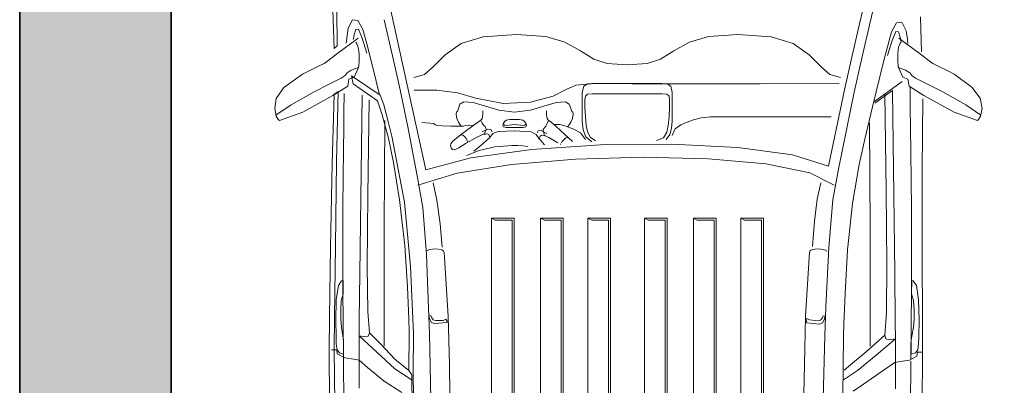
# Model space of a CAD drawing. Units: inches. Extents: x -5 to 482, y -460 to 66.
# Tile 7 of 31: x 33 to 91, y -351 to -329. Entities that reach past the tile are written whole.
import ezdxf

# ---------------------------------------------------------------- set-up
doc = ezdxf.new("R2010")
doc.units = ezdxf.units.IN
doc.header["$MEASUREMENT"] = 0
for name, color, linetype, lineweight in [('A-EQPM-VEHI', 8, 'Continuous', 13), ('A-WALL', 7, 'Continuous', 35), ('A-WALL-PATT', 152, 'Continuous', 13)]:
    doc.layers.add(name, color=color, linetype=linetype, lineweight=lineweight)

msp = doc.modelspace()

# ---------------------------------------------------------------- hatches: boundary and pattern name
at = {"layer": 'A-WALL-PATT'}
h = msp.add_hatch(color=256, dxfattribs=at)
h.dxf.hatch_style = 1
h.paths.add_polyline_path([(149.377, -412.849), (144.377, -412.849), (144.377, -283.849), (144.377, -279.349), (133.877, -279.349), (133.877, -283.849), (139.877, -283.849), (139.877, -412.849), (133.51, -412.849), (133.51, -413.916), (102.652, -413.916), (102.652, -421.02), (133.51, -421.02), (133.51, -421.849), (149.377, -421.849)])
h.paths.add_polyline_path([(226.054, -412.849), (218.877, -412.849), (218.877, -350.849), (262.877, -350.849), (262.877, -386.849), (267.377, -386.849), (267.377, -283.849), (270.377, -283.849), (270.377, -279.349), (244.877, -279.349), (244.877, -283.849), (262.877, -283.849), (262.877, -346.349), (218.877, -346.349), (218.877, -283.849), (220.877, -283.849), (220.877, -279.349), (214.377, -279.349), (214.377, -283.849), (214.377, -412.849), (209.377, -412.849), (209.377, -421.849), (226.054, -421.849)])
h.paths.add_polyline_path([(315.815, -412.849), (250.054, -412.849), (250.054, -421.849), (315.815, -421.849)])
h.paths.add_polyline_path([(430.377, -378.349), (421.377, -378.349), (421.377, -412.849), (375.815, -412.849), (375.815, -421.849), (430.377, -421.849)])
h.paths.add_polyline_path([(78.691, -413.916), (47.68, -413.916), (47.68, -412.849), (41.877, -412.849), (41.877, -283.849), (109.877, -283.849), (109.877, -279.349), (41.877, -279.349), (41.877, -241.849), (32.877, -241.849), (32.877, -421.849), (47.68, -421.849), (47.68, -421.02), (78.691, -421.02)])
h.paths.add_polyline_path([(41.877, -144.349), (154.377, -144.349), (154.377, -137.849), (149.877, -137.849), (149.877, -139.849), (41.877, -139.849), (41.877, -97.849), (32.877, -97.849), (32.877, -181.849), (41.877, -181.849)])
h.paths.add_polyline_path([(430.377, -241.849), (421.377, -241.849), (421.377, -279.349), (309.377, -279.349), (309.377, -170.349), (304.877, -170.349), (304.877, -279.349), (294.377, -279.349), (294.377, -283.849), (421.377, -283.849), (421.377, -318.349), (430.377, -318.349)])
h.paths.add_polyline_path([(430.377, -119.849), (421.377, -119.849), (421.377, -139.849), (419.377, -139.849), (419.377, -144.349), (421.377, -144.349), (421.377, -181.849), (430.377, -181.849)])
h.paths.add_polyline_path([(395.377, -139.849), (377.377, -139.849), (377.377, -75.849), (421.377, -75.849), (421.377, -95.849), (430.377, -95.849), (430.377, -45.599), (421.377, -45.599), (421.377, -71.349), (377.377, -71.349), (377.377, -22.849), (372.877, -22.849), (372.877, -139.849), (242.877, -139.849), (242.877, -137.849), (238.377, -137.849), (238.377, -144.349), (304.877, -144.349), (304.877, -146.349), (309.377, -146.349), (309.377, -144.349), (395.377, -144.349)])
h.paths.add_polyline_path([(65.877, 13.151), (32.877, 13.151), (32.877, -37.849), (41.877, -37.849), (41.877, 4.151), (65.877, 4.151)])
h.paths.add_polyline_path([(166.377, 13.151), (125.877, 13.151), (125.877, 4.151), (149.877, 4.151), (149.877, -113.849), (154.377, -113.849), (154.377, 4.151), (166.377, 4.151)])
h.paths.add_polyline_path([(277.877, 13.151), (226.377, 13.151), (226.377, 4.151), (238.377, 4.151), (238.377, -113.849), (242.877, -113.849), (242.877, 4.151), (277.877, 4.151)])
h.paths.add_polyline_path([(430.377, 13.151), (337.877, 13.151), (337.877, 4.151), (372.877, 4.151), (372.877, 1.151), (377.377, 1.151), (377.377, 4.151), (421.377, 4.151), (421.377, -21.599), (430.377, -21.599)])

# ---------------------------------------------------------------- linework, layer by layer
at = {"layer": 'A-EQPM-VEHI'}
for p, q in [((51.501, -329.276), (51.446, -328.108)), ((54.877, -328.542), (56.991, -338.198)), ((82.759, -329.511), (82.972, -328.603)), ((83.612, -328.412), (83.382, -329.41)), ((51.711, -328.752), (51.727, -330.829)), ((86.365, -329.094), (86.429, -331.173)), ((51.545, -330.986), (51.501, -329.276)), ((52.377, -329.78), (52.336, -330.066)), ((52.377, -329.78), (52.648, -329.267)), ((52.648, -329.267), (52.956, -329.307)), ((52.956, -329.307), (53.25, -329.847)), ((54.521, -329.266), (55.012, -331.413)), ((82.301, -331.49), (82.759, -329.511)), ((83.382, -329.41), (82.89, -331.556)), ((84.946, -329.451), (84.653, -329.99)), ((85.255, -329.411), (84.946, -329.451)), ((85.526, -329.923), (85.255, -329.411)), ((52.969, -330.36), (51.685, -331.319)), ((52.301, -330.358), (52.27, -330.656)), ((52.336, -330.066), (52.301, -330.358)), ((52.744, -330.168), (52.693, -330.377)), ((52.847, -329.847), (52.744, -330.168)), ((53.005, -329.824), (52.847, -329.847)), ((53.215, -330.362), (53.005, -329.824)), ((53.485, -331.257), (53.215, -330.362)), ((53.25, -329.847), (53.492, -330.702)), ((59.102, -330.69), (60.395, -330.28)), ((60.395, -330.28), (62.381, -330.141)), ((62.381, -330.141), (64.123, -330.258)), ((64.123, -330.258), (65.258, -330.594)), ((72.65, -330.594), (73.785, -330.258)), ((73.785, -330.258), (75.527, -330.141)), ((75.527, -330.141), (77.513, -330.28)), ((77.513, -330.28), (78.806, -330.69)), ((84.653, -329.99), (84.177, -331.772)), ((84.688, -330.505), (84.898, -329.968)), ((84.898, -329.968), (85.056, -329.99)), ((85.056, -329.99), (85.159, -330.311)), ((85.089, -330.36), (86.373, -331.319)), ((85.159, -330.311), (85.21, -330.52)), ((85.526, -329.923), (85.562, -330.172)), ((85.562, -330.172), (85.593, -330.425)), ((51.727, -330.829), (51.545, -330.986)), ((52.693, -330.377), (52.679, -330.451)), ((52.835, -330.595), (52.887, -330.666)), ((52.887, -330.666), (52.984, -330.893)), ((52.984, -330.893), (53.036, -331.3)), ((53.492, -330.702), (53.846, -332.115)), ((58.141, -331.359), (59.102, -330.69)), ((65.258, -330.594), (66.182, -331.125)), ((71.727, -331.125), (72.65, -330.594)), ((78.806, -330.69), (79.767, -331.359)), ((84.418, -331.401), (84.688, -330.505)), ((85.075, -330.893), (85.022, -331.3)), ((85.172, -330.666), (85.075, -330.893)), ((85.224, -330.595), (85.172, -330.666)), ((85.21, -330.52), (85.224, -330.595)), ((85.593, -330.425), (85.621, -330.682)), ((51.685, -331.319), (51.096, -331.763)), ((53.036, -331.3), (53.028, -331.733)), ((55.012, -331.413), (55.466, -333.44)), ((57.427, -332.063), (58.141, -331.359)), ((66.182, -331.125), (66.981, -331.617)), ((70.927, -331.617), (71.727, -331.125)), ((79.767, -331.359), (80.481, -332.063)), ((81.864, -333.428), (82.301, -331.49)), ((85.022, -331.3), (85.031, -331.733)), ((86.373, -331.319), (86.963, -331.763)), ((50.669, -332.009), (50.101, -332.288)), ((50.954, -331.871), (50.669, -332.009)), ((51.096, -331.763), (50.954, -331.871)), ((53.003, -332.106), (52.57, -332.273)), ((53.003, -332.106), (52.734, -332.677)), ((53.011, -332.009), (53.003, -332.106)), ((53.028, -331.733), (53.011, -332.009)), ((53.846, -332.115), (54.237, -333.736)), ((56.914, -332.535), (57.427, -332.063)), ((66.981, -331.617), (67.763, -331.878)), ((67.763, -331.878), (68.954, -331.955)), ((68.954, -331.955), (70.145, -331.878)), ((70.145, -331.878), (70.927, -331.617)), ((80.481, -332.063), (80.995, -332.535)), ((82.89, -331.556), (82.436, -333.584)), ((84.177, -331.772), (83.529, -334.456)), ((85.031, -331.733), (85.047, -332.009)), ((85.047, -332.009), (85.056, -332.106)), ((85.056, -332.106), (85.325, -332.677)), ((85.056, -332.106), (85.489, -332.273)), ((86.963, -331.763), (87.104, -331.871)), ((87.104, -331.871), (87.389, -332.008)), ((87.389, -332.008), (87.958, -332.287)), ((49.678, -332.509), (48.571, -333.307)), ((50.101, -332.288), (49.678, -332.509)), ((52.197, -332.576), (51.974, -332.745)), ((52.316, -332.432), (52.197, -332.576)), ((52.57, -332.273), (52.316, -332.432)), ((52.734, -332.677), (52.432, -332.811)), ((52.573, -332.611), (54.277, -333.756)), ((52.69, -333.08), (52.573, -332.611)), ((56.293, -332.697), (56.914, -332.535)), ((80.995, -332.535), (81.616, -332.697)), ((85.325, -332.677), (85.627, -332.811)), ((85.489, -332.273), (85.742, -332.432)), ((85.742, -332.432), (85.862, -332.576)), ((85.862, -332.576), (86.085, -332.745)), ((87.958, -332.287), (88.381, -332.509)), ((88.381, -332.509), (89.411, -333.269)), ((51.223, -333.114), (50.367, -333.56)), ((51.58, -332.944), (51.223, -333.114)), ((51.482, -333.765), (52.365, -333.214)), ((51.974, -332.745), (51.58, -332.944)), ((52.365, -333.214), (52.432, -332.811)), ((54.121, -334.081), (52.69, -333.08)), ((65.908, -333.15), (65.338, -333.419)), ((67.024, -333.06), (65.908, -333.15)), ((66.369, -333.212), (66.285, -333.597)), ((66.587, -333.077), (66.369, -333.212)), ((66.89, -333.061), (66.587, -333.077)), ((71.018, -333.061), (66.89, -333.061)), ((69.258, -333.072), (67.024, -333.06)), ((72.651, -333.079), (69.258, -333.072)), ((71.321, -333.077), (71.018, -333.061)), ((71.539, -333.212), (71.321, -333.077)), ((71.623, -333.597), (71.539, -333.212)), ((76.859, -333.078), (72.651, -333.079)), ((81.536, -333.067), (76.859, -333.078)), ((85.291, -332.946), (83.645, -334.121)), ((85.694, -333.214), (85.627, -332.811)), ((86.577, -333.765), (85.694, -333.214)), ((85.749, -333.232), (85.762, -334.455)), ((86.085, -332.745), (86.479, -332.944)), ((86.479, -332.944), (86.836, -333.114)), ((86.836, -333.114), (87.691, -333.56)), ((89.411, -333.269), (89.915, -333.933)), ((48.571, -333.307), (48.105, -333.952)), ((50.367, -333.56), (48.996, -334.324)), ((49.695, -334.768), (51.482, -333.765)), ((51.438, -337.84), (51.545, -333.691)), ((51.545, -333.691), (51.792, -333.543)), ((51.792, -333.543), (51.695, -337.715)), ((52.141, -333.662), (52.13, -334.738)), ((53.221, -333.746), (53.134, -339.877)), ((54.277, -333.756), (54.505, -334.336)), ((55.466, -333.44), (55.941, -335.733)), ((57.641, -333.457), (56.294, -333.457)), ((58.87, -333.613), (57.641, -333.457)), ((59.974, -333.925), (58.87, -333.613)), ((64.553, -333.821), (63.206, -334.171)), ((65.338, -333.419), (64.553, -333.821)), ((66.285, -333.597), (66.285, -335.29)), ((66.468, -333.818), (66.432, -334.037)), ((66.601, -333.701), (66.468, -333.818)), ((66.873, -333.666), (66.601, -333.701)), ((66.873, -333.666), (71.036, -333.666)), ((71.036, -333.666), (71.307, -333.701)), ((71.307, -333.701), (71.441, -333.818)), ((71.441, -333.818), (71.476, -334.037)), ((71.623, -335.29), (71.623, -333.597)), ((81.522, -335.051), (81.864, -333.428)), ((82.436, -333.584), (81.99, -335.718)), ((83.652, -334.237), (84.705, -333.476)), ((84.25, -333.684), (84.335, -339.434)), ((84.705, -333.476), (84.788, -339.678)), ((88.363, -334.768), (86.577, -333.765)), ((87.691, -333.56), (89.062, -334.324)), ((48.105, -333.952), (48.029, -334.547)), ((48.996, -334.324), (48.096, -334.95)), ((53.638, -334.031), (53.555, -339.704)), ((54.395, -334.921), (54.121, -334.081)), ((54.505, -334.336), (54.786, -335.391)), ((58.935, -334.555), (59.023, -334.293)), ((59.023, -334.293), (59.257, -334.156)), ((59.257, -334.156), (59.799, -334.193)), ((59.799, -334.193), (60.543, -334.402)), ((61.588, -334.25), (59.974, -333.925)), ((60.543, -334.402), (61.335, -334.646)), ((63.206, -334.171), (61.588, -334.25)), ((63.995, -334.402), (63.203, -334.646)), ((64.739, -334.193), (63.995, -334.402)), ((65.282, -334.156), (64.739, -334.193)), ((65.516, -334.293), (65.282, -334.156)), ((65.603, -334.555), (65.516, -334.293)), ((66.432, -334.037), (66.442, -334.464)), ((71.476, -334.037), (71.467, -334.464)), ((83.529, -334.456), (83.074, -336.371)), ((85.762, -334.455), (85.773, -335.747)), ((86.509, -333.977), (86.463, -338.174)), ((89.062, -334.324), (89.963, -334.95)), ((89.915, -333.933), (90.03, -334.547)), ((48.029, -334.547), (48.113, -334.998)), ((48.113, -334.998), (48.235, -335.203)), ((48.297, -335.252), (49.695, -334.768)), ((52.13, -334.738), (52.127, -335.745)), ((54.624, -335.731), (54.395, -334.921)), ((58.789, -334.884), (58.819, -334.749)), ((58.828, -335.143), (58.789, -334.884)), ((58.819, -334.749), (58.87, -334.719)), ((58.87, -334.719), (58.935, -334.555)), ((60.377, -334.918), (60.341, -335.14)), ((60.386, -334.685), (60.377, -334.918)), ((61.335, -334.646), (62.269, -334.763)), ((63.203, -334.646), (62.269, -334.763)), ((64.152, -334.685), (64.163, -334.917)), ((64.163, -334.917), (64.201, -335.139)), ((65.668, -334.719), (65.603, -334.555)), ((65.719, -334.749), (65.668, -334.719)), ((65.71, -335.143), (65.75, -334.884)), ((65.75, -334.884), (65.719, -334.749)), ((66.442, -334.464), (66.472, -335.042)), ((66.472, -335.042), (66.527, -335.549)), ((71.437, -335.042), (71.381, -335.549)), ((71.467, -334.464), (71.437, -335.042)), ((73.892, -335.044), (73.355, -335.096)), ((81.072, -335.044), (73.892, -335.044)), ((89.761, -335.252), (88.363, -334.768)), ((89.945, -334.998), (89.823, -335.203)), ((90.03, -334.547), (89.945, -334.998)), ((48.235, -335.203), (48.297, -335.252)), ((54.56, -335.254), (54.521, -341.596)), ((54.786, -335.391), (54.98, -336.191)), ((57.477, -335.434), (56.762, -335.382)), ((57.497, -335.462), (57.477, -335.434)), ((57.569, -335.519), (57.497, -335.462)), ((57.711, -335.564), (57.569, -335.519)), ((57.987, -335.585), (57.711, -335.564)), ((58.479, -335.597), (57.987, -335.585)), ((59.229, -335.6), (58.479, -335.597)), ((58.933, -335.364), (58.828, -335.143)), ((59.03, -335.514), (58.933, -335.364)), ((59.093, -335.59), (59.03, -335.514)), ((59.154, -335.617), (59.093, -335.59)), ((59.229, -335.6), (59.154, -335.617)), ((59.336, -335.566), (59.229, -335.6)), ((59.505, -335.546), (59.336, -335.566)), ((59.773, -335.557), (59.505, -335.546)), ((60.119, -335.333), (59.711, -335.633)), ((60.203, -335.278), (60.119, -335.333)), ((60.236, -335.278), (60.203, -335.278)), ((60.242, -335.287), (60.236, -335.278)), ((60.341, -335.14), (60.242, -335.287)), ((60.277, -335.289), (60.339, -335.421)), ((60.339, -335.421), (60.424, -335.528)), ((60.424, -335.528), (60.511, -335.621)), ((60.511, -335.621), (60.565, -335.709)), ((61.567, -335.551), (61.613, -335.411)), ((61.607, -335.639), (61.567, -335.551)), ((61.607, -335.481), (61.613, -335.411)), ((61.659, -335.544), (61.607, -335.481)), ((61.613, -335.411), (61.695, -335.292)), ((61.768, -335.557), (61.659, -335.544)), ((61.695, -335.292), (61.784, -335.241)), ((61.925, -335.53), (61.768, -335.557)), ((61.784, -335.241), (61.872, -335.221)), ((61.872, -335.221), (61.981, -335.206)), ((62.104, -335.507), (61.925, -335.53)), ((61.981, -335.206), (62.12, -335.198)), ((62.278, -335.497), (62.104, -335.507)), ((62.12, -335.198), (62.269, -335.195)), ((62.269, -335.195), (62.418, -335.198)), ((62.448, -335.507), (62.278, -335.497)), ((62.418, -335.198), (62.558, -335.206)), ((62.618, -335.53), (62.448, -335.507)), ((62.558, -335.206), (62.667, -335.221)), ((62.77, -335.557), (62.618, -335.53)), ((62.667, -335.221), (62.755, -335.241)), ((62.755, -335.241), (62.843, -335.292)), ((62.88, -335.544), (62.77, -335.557)), ((62.843, -335.292), (62.926, -335.411)), ((62.931, -335.481), (62.88, -335.544)), ((62.926, -335.411), (62.972, -335.551)), ((62.926, -335.411), (62.931, -335.481)), ((62.972, -335.551), (62.931, -335.639)), ((64.119, -335.597), (64.031, -335.713)), ((64.2, -335.445), (64.119, -335.597)), ((64.264, -335.29), (64.2, -335.445)), ((64.201, -335.139), (64.299, -335.29)), ((64.299, -335.29), (64.305, -335.28)), ((64.305, -335.28), (64.339, -335.282)), ((64.339, -335.282), (64.42, -335.341)), ((64.42, -335.341), (64.715, -335.605)), ((64.644, -335.488), (64.944, -335.494)), ((64.715, -335.605), (65.231, -336.066)), ((64.944, -335.494), (65.172, -335.548)), ((65.172, -335.548), (65.309, -335.6)), ((65.309, -335.6), (65.384, -335.617)), ((65.384, -335.617), (65.445, -335.59)), ((65.445, -335.59), (65.508, -335.514)), ((65.508, -335.514), (65.605, -335.364)), ((65.605, -335.364), (65.71, -335.143)), ((66.285, -335.29), (66.33, -335.813)), ((66.527, -335.549), (66.604, -335.912)), ((71.381, -335.549), (71.3, -335.947)), ((71.594, -335.723), (71.623, -335.29)), ((72.148, -335.513), (71.808, -335.759)), ((72.513, -335.356), (72.148, -335.513)), ((72.894, -335.217), (72.513, -335.356)), ((73.355, -335.096), (72.894, -335.217)), ((81.115, -337.014), (81.522, -335.051)), ((83.343, -335.397), (83.382, -341.702)), ((89.823, -335.203), (89.761, -335.252)), ((52.127, -335.745), (52.108, -336.966)), ((54.771, -336.306), (54.624, -335.731)), ((54.98, -336.191), (55.72, -340.115)), ((55.941, -335.733), (56.491, -338.549)), ((59.037, -336.129), (58.571, -336.505)), ((59.711, -335.633), (59.037, -336.129)), ((59.066, -336.124), (59.133, -336.106)), ((59.133, -336.106), (59.202, -336.128)), ((59.202, -336.128), (59.286, -336.214)), ((59.286, -336.214), (59.382, -336.337)), ((59.971, -336.29), (60.41, -336.065)), ((60.682, -335.777), (60.34, -335.923)), ((60.41, -336.065), (60.422, -336.069)), ((60.422, -336.069), (60.463, -336.073)), ((60.463, -336.073), (60.54, -336.063)), ((60.492, -335.989), (60.48, -336.043)), ((60.48, -336.043), (60.48, -336.06)), ((60.531, -335.899), (60.492, -335.989)), ((60.57, -335.798), (60.531, -335.899)), ((60.54, -336.063), (60.64, -336.053)), ((60.565, -335.709), (60.57, -335.798)), ((60.64, -336.053), (60.732, -336.101)), ((60.859, -335.8), (60.682, -335.777)), ((60.732, -336.101), (60.789, -336.267)), ((60.969, -336.038), (60.789, -336.267)), ((60.927, -335.928), (60.859, -335.8)), ((61.29, -335.914), (60.969, -336.038)), ((62.295, -335.877), (61.29, -335.914)), ((61.768, -335.67), (61.607, -335.639)), ((62.77, -335.67), (61.768, -335.67)), ((62.243, -335.877), (63.244, -335.931)), ((62.931, -335.639), (62.77, -335.67)), ((63.244, -335.931), (63.554, -336.088)), ((63.554, -336.088), (63.72, -336.343)), ((63.599, -335.998), (63.675, -335.874)), ((63.675, -335.874), (63.852, -335.86)), ((63.785, -336.181), (63.72, -336.343)), ((63.88, -336.137), (63.785, -336.181)), ((63.852, -335.86), (64.187, -336.024)), ((63.979, -336.153), (63.88, -336.137)), ((63.972, -335.798), (63.963, -335.887)), ((63.963, -335.887), (63.997, -335.989)), ((64.031, -335.713), (63.972, -335.798)), ((64.055, -336.167), (63.979, -336.153)), ((63.997, -335.989), (64.031, -336.082)), ((64.031, -336.082), (64.04, -336.136)), ((64.04, -336.136), (64.04, -336.153)), ((64.096, -336.165), (64.055, -336.167)), ((64.109, -336.162), (64.096, -336.165)), ((64.294, -336.265), (64.109, -336.162)), ((65.231, -336.066), (65.705, -336.502)), ((65.411, -335.642), (65.786, -335.78)), ((65.786, -335.78), (66.172, -335.999)), ((66.172, -335.999), (66.478, -336.397)), ((66.33, -335.813), (66.503, -336.237)), ((66.604, -335.912), (66.763, -336.244)), ((71.3, -335.947), (71.111, -336.283)), ((71.27, -336.379), (71.487, -336.094)), ((71.487, -336.094), (71.594, -335.723)), ((71.808, -335.759), (71.616, -336.149)), ((81.99, -335.718), (81.487, -338.241)), ((85.773, -335.747), (85.795, -337.11)), ((55.072, -337.759), (54.771, -336.306)), ((58.479, -336.641), (58.46, -336.773)), ((58.46, -336.773), (58.499, -336.89)), ((58.571, -336.505), (58.479, -336.641)), ((58.957, -336.88), (59.399, -336.609)), ((59.382, -336.337), (59.452, -336.453)), ((59.399, -336.609), (59.971, -336.29)), ((59.452, -336.453), (59.467, -336.561)), ((60.416, -336.607), (60.029, -336.937)), ((60.789, -336.267), (60.416, -336.607)), ((61.088, -336.829), (62.122, -336.749)), ((62.122, -336.749), (62.457, -336.75)), ((62.457, -336.75), (62.752, -336.762)), ((62.752, -336.762), (63.063, -336.798)), ((63.262, -336.987), (67.369, -336.714)), ((63.72, -336.343), (63.821, -336.455)), ((63.821, -336.455), (63.925, -336.569)), ((63.925, -336.569), (64.049, -336.703)), ((64.539, -336.41), (64.294, -336.265)), ((64.827, -336.588), (64.539, -336.41)), ((64.964, -336.669), (65.013, -336.666)), ((64.981, -336.668), (64.964, -336.669)), ((64.997, -336.667), (64.981, -336.668)), ((65.013, -336.666), (64.997, -336.667)), ((65.099, -336.516), (65.052, -336.587)), ((65.158, -336.444), (65.099, -336.516)), ((65.223, -336.369), (65.158, -336.444)), ((65.312, -336.288), (65.223, -336.369)), ((65.382, -336.269), (65.312, -336.288)), ((65.448, -336.291), (65.382, -336.269)), ((66.503, -336.237), (66.861, -336.518)), ((66.763, -336.244), (67.078, -336.463)), ((67.369, -336.714), (71.59, -336.67)), ((71.111, -336.283), (70.69, -336.457)), ((71.59, -336.67), (75.522, -336.861)), ((83.074, -336.371), (82.737, -337.876)), ((52.108, -336.966), (52.07, -340.371)), ((58.499, -336.89), (58.582, -336.98)), ((58.582, -336.98), (58.725, -336.996)), ((58.725, -336.996), (58.957, -336.88)), ((59.404, -337.34), (60.156, -337.041)), ((59.669, -337.483), (63.262, -336.987)), ((60.029, -336.937), (59.851, -337.086)), ((60.156, -337.041), (61.088, -336.829)), ((75.522, -336.861), (78.765, -337.291)), ((78.765, -337.291), (80.918, -337.968)), ((80.918, -337.968), (81.115, -337.014)), ((85.795, -337.11), (85.833, -340.514)), ((51.342, -342.782), (51.438, -337.84)), ((51.695, -337.715), (51.622, -342.708)), ((55.433, -339.982), (55.072, -337.759)), ((56.991, -338.198), (59.669, -337.483)), ((62.093, -337.877), (58.856, -338.397)), ((65.888, -337.556), (62.093, -337.877)), ((69.897, -337.44), (65.888, -337.556)), ((73.78, -337.532), (69.897, -337.44)), ((77.195, -337.839), (73.78, -337.532)), ((79.798, -338.364), (77.195, -337.839)), ((82.737, -337.876), (82.326, -340.195)), ((56.491, -338.549), (56.819, -340.434)), ((58.856, -338.397), (56.519, -339.112)), ((81.249, -339.112), (79.798, -338.364)), ((81.487, -338.241), (81.169, -339.966)), ((86.463, -338.174), (86.464, -343.144)), ((57.425, -338.972), (57.653, -340.004)), ((80.454, -338.972), (80.243, -339.939)), ((53.555, -339.704), (53.519, -343.89)), ((84.335, -339.434), (84.376, -343.789)), ((84.788, -339.678), (84.842, -344.319)), ((53.134, -339.877), (53.074, -344.362)), ((55.747, -342.679), (55.433, -339.982)), ((55.72, -340.115), (56.091, -343.938)), ((57.653, -340.004), (57.847, -341.392)), ((80.243, -339.939), (80.078, -341.249)), ((81.169, -339.966), (80.93, -342.811)), ((82.326, -340.195), (82.033, -342.953)), ((52.07, -340.371), (52.068, -343.738)), ((56.819, -340.434), (57.028, -343.23)), ((85.833, -340.514), (85.835, -343.881)), ((57.847, -341.392), (57.971, -342.796)), ((61.121, -341.174), (60.891, -341.062)), ((62.245, -341.062), (60.891, -341.062)), ((60.892, -376.546), (60.892, -341.062)), ((62.122, -341.174), (61.121, -341.174)), ((62.109, -375.982), (62.122, -341.174)), ((62.244, -341.062), (62.244, -376.546)), ((62.245, -341.062), (62.245, -376.546)), ((64.034, -341.174), (63.805, -341.062)), ((65.159, -341.062), (63.805, -341.062)), ((63.806, -376.546), (63.806, -341.062)), ((65.036, -341.174), (64.034, -341.174)), ((65.023, -375.982), (65.036, -341.174)), ((65.157, -341.062), (65.157, -376.546)), ((65.159, -341.062), (65.159, -376.546)), ((66.844, -341.174), (66.614, -341.062)), ((67.968, -341.062), (66.614, -341.062)), ((66.616, -376.546), (66.616, -341.062)), ((67.845, -341.174), (66.844, -341.174)), ((67.833, -375.982), (67.845, -341.174)), ((67.967, -341.062), (67.967, -376.546)), ((67.968, -341.062), (67.968, -376.546)), ((70.205, -341.174), (69.976, -341.062)), ((71.33, -341.062), (69.976, -341.062)), ((69.977, -376.546), (69.977, -341.062)), ((71.207, -341.174), (70.205, -341.174)), ((71.194, -375.982), (71.207, -341.174)), ((71.329, -341.062), (71.329, -376.546)), ((71.33, -341.062), (71.33, -376.546)), ((73.119, -341.174), (72.89, -341.062)), ((74.243, -341.062), (72.89, -341.062)), ((72.891, -376.546), (72.891, -341.062)), ((74.121, -341.174), (73.119, -341.174)), ((74.108, -375.982), (74.121, -341.174)), ((74.242, -341.062), (74.242, -376.546)), ((74.243, -341.062), (74.243, -376.546)), ((75.7, -376.546), (75.7, -341.062)), ((75.93, -341.174), (75.7, -341.062)), ((75.7, -341.062), (77.053, -341.062)), ((76.932, -341.174), (75.93, -341.174)), ((76.918, -375.982), (76.932, -341.174)), ((77.053, -341.062), (77.053, -376.546)), ((80.078, -341.249), (79.954, -342.744)), ((54.521, -341.596), (54.518, -346.619)), ((83.382, -341.702), (83.383, -346.656)), ((51.274, -346.976), (51.342, -342.782)), ((51.622, -342.708), (51.576, -346.953)), ((55.915, -345.149), (55.747, -342.679)), ((57.028, -343.23), (57.164, -346.404)), ((57.22, -342.927), (57.033, -343.031)), ((57.575, -342.888), (57.22, -342.927)), ((57.897, -342.919), (57.575, -342.888)), ((57.979, -342.959), (57.897, -342.919)), ((58.045, -343.027), (57.979, -342.959)), ((58.075, -343.108), (58.045, -343.027)), ((58.318, -346.891), (58.075, -343.108)), ((79.536, -346.891), (79.771, -343.108)), ((79.771, -343.108), (79.801, -343.027)), ((79.801, -343.027), (79.867, -342.959)), ((79.867, -342.959), (79.95, -342.919)), ((79.95, -342.919), (80.271, -342.888)), ((80.271, -342.888), (80.627, -342.927)), ((80.627, -342.927), (80.813, -343.031)), ((80.93, -342.811), (80.757, -346.334)), ((82.033, -342.953), (81.898, -345.546)), ((86.464, -343.144), (86.486, -347.294)), ((52.068, -343.738), (52.075, -345.261)), ((84.376, -343.789), (84.354, -346.676)), ((53.074, -344.362), (53.039, -347.115)), ((53.519, -343.89), (53.547, -346.609)), ((56.091, -343.938), (56.261, -347.911)), ((84.842, -344.319), (84.87, -347.228)), ((85.835, -343.881), (85.828, -345.405)), ((51.992, -344.793), (51.805, -345.065)), ((52.088, -344.774), (51.992, -344.793)), ((52.096, -345.566), (52.088, -344.774)), ((85.84, -345.566), (85.848, -344.774)), ((85.848, -344.774), (85.943, -344.793)), ((85.943, -344.793), (86.131, -345.065)), ((51.805, -345.065), (51.673, -345.91)), ((51.976, -345.955), (52.096, -345.566)), ((52.075, -345.261), (52.108, -349.325)), ((55.99, -347.062), (55.915, -345.149)), ((81.898, -345.546), (81.822, -347.369)), ((85.828, -345.405), (85.795, -349.469)), ((85.96, -345.955), (85.84, -345.566)), ((86.131, -345.065), (86.262, -345.91)), ((51.673, -345.91), (51.65, -347.124)), ((51.943, -346.529), (51.976, -345.955)), ((85.992, -346.529), (85.96, -345.955)), ((86.262, -345.91), (86.285, -347.124)), ((51.945, -347.046), (51.943, -346.529)), ((53.547, -346.609), (53.653, -347.881)), ((54.518, -346.619), (54.524, -348.663)), ((57.164, -346.404), (57.213, -347.914)), ((80.757, -346.334), (80.69, -348.058)), ((83.383, -346.656), (83.377, -348.663)), ((84.354, -346.676), (84.25, -348.024)), ((85.991, -347.046), (85.992, -346.529)), ((51.247, -348.881), (51.274, -346.976)), ((51.576, -346.953), (51.559, -348.88)), ((51.65, -347.124), (51.663, -348.12)), ((51.988, -347.557), (51.945, -347.046)), ((53.039, -347.115), (53.028, -348.051)), ((56.007, -347.83), (55.99, -347.062)), ((57.177, -346.872), (57.294, -346.848)), ((57.232, -347.086), (57.177, -346.872)), ((57.331, -347.267), (57.232, -347.086)), ((57.294, -346.848), (57.343, -346.986)), ((57.508, -347.331), (57.331, -347.267)), ((57.343, -346.986), (57.436, -347.101)), ((57.436, -347.101), (57.574, -347.139)), ((58.263, -347.257), (57.508, -347.331)), ((57.574, -347.139), (57.734, -347.147)), ((57.734, -347.147), (58.03, -347.139)), ((58.03, -347.139), (58.187, -347.07)), ((58.187, -347.07), (58.246, -347.158)), ((58.246, -347.158), (58.263, -347.228)), ((58.263, -347.228), (58.263, -347.257)), ((58.394, -349.773), (58.318, -346.891)), ((79.476, -349.773), (79.536, -346.891)), ((79.614, -347.018), (79.575, -347.126)), ((79.575, -347.126), (79.595, -347.233)), ((79.595, -347.233), (79.615, -347.282)), ((79.79, -347.108), (79.614, -347.018)), ((79.615, -347.282), (80.37, -347.357)), ((80.124, -347.152), (79.79, -347.108)), ((80.304, -347.165), (80.124, -347.152)), ((80.442, -347.127), (80.304, -347.165)), ((80.37, -347.357), (80.547, -347.294)), ((80.536, -347.012), (80.442, -347.127)), ((80.585, -346.874), (80.536, -347.012)), ((80.547, -347.294), (80.647, -347.112)), ((80.701, -346.898), (80.585, -346.874)), ((80.647, -347.112), (80.701, -346.898)), ((84.87, -347.228), (84.878, -348.236)), ((85.947, -347.557), (85.991, -347.046)), ((86.285, -347.124), (86.272, -348.12)), ((86.486, -347.294), (86.5, -349.032)), ((52.069, -348.079), (51.988, -347.557)), ((53.653, -347.881), (53.58, -348.082)), ((53.653, -347.881), (54.326, -348.554)), ((55.987, -350.117), (56.007, -347.83)), ((81.822, -347.369), (81.798, -348.058)), ((85.866, -348.079), (85.947, -347.557)), ((51.663, -348.12), (51.676, -348.534)), ((52.113, -348.318), (52.069, -348.079)), ((52.113, -349.142), (52.113, -348.318)), ((53.028, -348.051), (54.087, -349.031)), ((53.391, -348.119), (53.028, -348.051)), ((53.028, -348.051), (53.041, -351.173)), ((53.58, -348.082), (53.391, -348.119)), ((56.261, -347.911), (56.245, -350.247)), ((57.213, -347.914), (57.291, -351.814)), ((80.69, -348.058), (80.592, -351.787)), ((81.798, -348.058), (81.767, -351.619)), ((84.25, -348.024), (83.136, -349.004)), ((84.878, -348.236), (83.744, -349.198)), ((84.25, -348.024), (84.323, -348.236)), ((84.323, -348.236), (84.513, -348.293)), ((84.513, -348.293), (84.878, -348.236)), ((84.878, -348.236), (84.888, -351.213)), ((85.822, -348.318), (85.866, -348.079)), ((85.822, -349.142), (85.822, -348.318)), ((86.272, -348.12), (86.26, -348.534)), ((51.274, -352.085), (51.247, -348.881)), ((51.705, -348.888), (51.403, -348.881)), ((51.559, -348.88), (51.586, -352.081)), ((51.676, -348.534), (51.729, -348.898)), ((51.739, -349.123), (51.705, -348.888)), ((51.729, -348.898), (51.869, -349.077)), ((51.869, -349.077), (52.113, -349.142)), ((54.087, -349.031), (55.152, -350.016)), ((54.326, -348.554), (55.145, -349.437)), ((83.136, -349.004), (82.217, -349.788)), ((86.067, -349.077), (85.822, -349.142)), ((86.207, -348.898), (86.067, -349.077)), ((86.164, -349.267), (86.198, -349.032)), ((86.198, -349.032), (86.488, -349.032)), ((86.26, -348.534), (86.207, -348.898)), ((86.473, -352.232), (86.5, -349.032)), ((52.188, -349.358), (51.739, -349.123)), ((52.108, -349.325), (52.134, -354.234)), ((52.726, -349.453), (52.188, -349.358)), ((53.041, -349.508), (52.726, -349.453)), ((53.531, -349.937), (53.041, -349.508)), ((55.145, -349.437), (55.987, -350.117)), ((83.744, -349.198), (82.621, -350.12)), ((84.158, -350.112), (84.844, -349.638)), ((84.844, -349.638), (85.164, -349.587)), ((85.164, -349.587), (85.71, -349.498)), ((85.71, -349.498), (86.164, -349.267)), ((85.799, -349.56), (85.773, -354.469)), ((54.515, -350.745), (53.531, -349.937)), ((55.152, -350.016), (56.176, -350.692)), ((56.17, -350.375), (55.987, -350.117)), ((56.245, -350.247), (56.261, -351.733)), ((58.428, -351.511), (58.394, -349.773)), ((79.451, -351.511), (79.476, -349.773)), ((82.621, -350.12), (81.801, -350.679)), ((82.217, -349.788), (81.834, -350.108)), ((82.99, -350.921), (84.158, -350.112)), ((55.564, -351.42), (54.515, -350.745)), ((56.182, -352.643), (56.17, -350.375)), ((82.371, -351.35), (82.99, -350.921))]:
    msp.add_line(p, q, dxfattribs=at)
at = {"layer": 'A-WALL'}
for p, q in [((32.877, 13.151), (32.877, -421.849)), ((41.877, -283.849), (41.877, -412.849))]:
    msp.add_line(p, q, dxfattribs=at)

doc.saveas('drawing.dxf')
